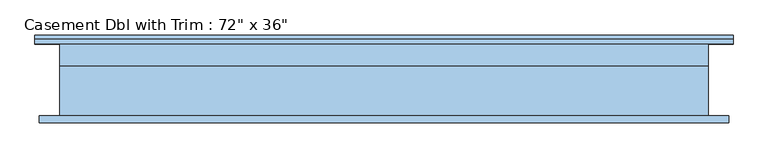
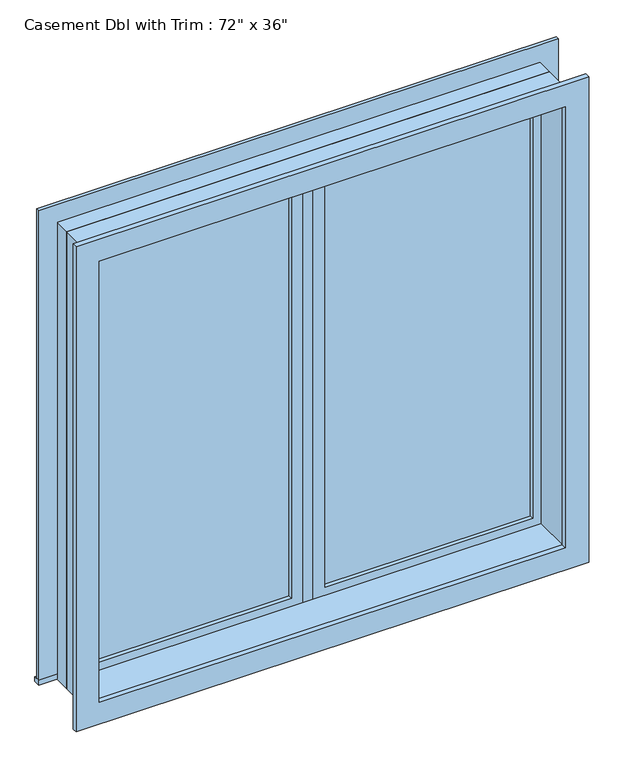
"""IFC4 building model written with IfcOpenShell, lengths in millimetres: window geometry."""

from ifc_helpers import new_model, si_unit, frame, origin, place, context, project, spatial, polyline, outline, extrude, source, transform, mapped, element, save


def window_b085ff8d(model_context):
    return source(origin(), model_context, "Body", "SweptSolid", [
        extrude(outline(polyline([(63.5, 85.725), (850.9, 85.725), (850.9, 73.025), (63.5, 73.025), (63.5, 85.725)])), frame((0.0, 0.0, 1282.7), z_axis=(0.0, 0.0, 1.0), x_axis=(1.0, 0.0, 0.0)), (0.0, 0.0, 1.0), 1701.8),
        extrude(outline(polyline([(3028.95, 19.05), (1238.25, 19.05), (1238.25, 895.35), (3028.95, 895.35), (3028.95, 19.05)]), holes=[polyline([(2984.5, 63.5), (2984.5, 850.9), (1282.7, 850.9), (1282.7, 63.5), (2984.5, 63.5)])]), frame((0.0, 57.15, 0.0), z_axis=(0.0, 1.0, 0.0), x_axis=(0.0, 0.0, 1.0)), (0.0, 0.0, 1.0), 44.45),
        extrude(outline(polyline([(19.05, 57.15), (-19.05, 57.15), (-19.05, 120.65), (19.05, 120.65), (19.05, 57.15)])), frame((0.0, 0.0, 1238.25), z_axis=(0.0, 0.0, 1.0), x_axis=(1.0, 0.0, 0.0)), (0.0, 0.0, 1.0), 1790.7),
        extrude(outline(polyline([(-984.25, 146.05), (984.25, 146.05), (984.25, 120.65), (-984.25, 120.65), (-984.25, 146.05)])), frame((0.0, 0.0, 1219.2), z_axis=(0.0, 0.0, 1.0), x_axis=(1.0, 0.0, 0.0)), (0.0, 0.0, 1.0), 19.05),
        extrude(outline(polyline([(3028.95, -895.35), (3028.95, 895.35), (1238.25, 895.35), (1238.25, 984.25), (3117.85, 984.25), (3117.85, -984.25), (1238.25, -984.25), (1238.25, -895.35), (3028.95, -895.35)])), frame((0.0, 120.65, 0.0), z_axis=(0.0, 1.0, 0.0), x_axis=(0.0, 0.0, 1.0)), (0.0, 0.0, 1.0), 12.7),
        extrude(outline(polyline([(3105.15, 971.55), (3105.15, -971.55), (1162.05, -971.55), (1162.05, 971.55), (3105.15, 971.55)]), holes=[polyline([(3016.25, 882.65), (1250.95, 882.65), (1250.95, -882.65), (3016.25, -882.65), (3016.25, 882.65)])]), frame((0.0, -101.6, 0.0), z_axis=(0.0, 1.0, 0.0), x_axis=(0.0, 0.0, 1.0)), (0.0, 0.0, 1.0), 19.05),
        extrude(outline(polyline([(-63.5, 73.025), (-850.9, 73.025), (-850.9, 85.725), (-63.5, 85.725), (-63.5, 73.025)])), frame((0.0, 0.0, 1282.7), z_axis=(0.0, 0.0, 1.0), x_axis=(1.0, 0.0, 0.0)), (0.0, 0.0, 1.0), 1701.8),
        extrude(outline(polyline([(3028.95, -895.35), (1238.25, -895.35), (1238.25, -19.05), (3028.95, -19.05), (3028.95, -895.35)]), holes=[polyline([(2984.5, -850.9), (2984.5, -63.5), (1282.7, -63.5), (1282.7, -850.9), (2984.5, -850.9)])]), frame((0.0, 57.15, 0.0), z_axis=(0.0, 1.0, 0.0), x_axis=(0.0, 0.0, 1.0)), (0.0, 0.0, 1.0), 44.45),
        extrude(outline(polyline([(3048.0, -914.4), (1219.2, -914.4), (1219.2, 914.4), (3048.0, 914.4), (3048.0, -914.4)]), holes=[polyline([(3016.25, -882.65), (3016.25, 882.65), (1250.95, 882.65), (1250.95, -882.65), (3016.25, -882.65)])]), frame((0.0, -82.55, 0.0), z_axis=(0.0, 1.0, 0.0), x_axis=(0.0, 0.0, 1.0)), (0.0, 0.0, 1.0), 139.7),
        extrude(outline(polyline([(3048.0, 914.4), (3048.0, -914.4), (1219.2, -914.4), (1219.2, 914.4), (3048.0, 914.4)]), holes=[polyline([(3028.95, 895.35), (1238.25, 895.35), (1238.25, -895.35), (3028.95, -895.35), (3028.95, 895.35)])]), frame((0.0, 57.15, 0.0), z_axis=(0.0, 1.0, 0.0), x_axis=(0.0, 0.0, 1.0)), (0.0, 0.0, 1.0), 63.5),
    ])


if __name__ == "__main__":
    model = new_model("IFC4")
    model_context = context("Model", 3, world=origin())
    ifc_project = project(units=[si_unit("LENGTHUNIT", "METRE", prefix="MILLI")], contexts=[model_context])
    site = spatial("IfcSite", under=ifc_project)
    building = spatial("IfcBuilding", under=site)
    placement = place(None, origin())
    window_shape = window_b085ff8d(model_context)
    element("IfcWindow", 1, ObjectType="Casement Dbl with Trim : 72\" x 36\"", at=placement, inside=building, context=model_context, shape_type="MappedRepresentation", body=[
        mapped(window_shape, transform((0.0, 0.0, 0.0), x_axis=(1.0, 0.0, 0.0), y_axis=(0.0, 1.0, 0.0), z_axis=(0.0, 0.0, 1.0))),
    ])
    save(model, "model.ifc")

# Revit data of these elements
# Type "Casement Dbl with Trim : 72\" x 36\""
#   Type Mark = "11"
#   Construction Type Id = "GSP4R"
#   Assembly Code = "B2020100"
#   Analytic Construction = "1/8 in Pilkington single glazing"
#   Visual Light Transmittance = 0.9
#   Solar Heat Gain Coefficient = 0.78
#   Heat Transfer Coefficient (U) = 0.6496 BTU/(h·ft²·°F)
#   Height = 6' - 0"
#   Default Sill Height = 4' - 0"
#   Trim Projection - Ext. = 0' - 0 1/2"
#   Trim Projection - Int. = 0' - 0 3/4"
#   Trim Width - Exterior = 0' - 3 1/2"
#   Trim Width - Interior = 0' - 3 1/2"
#   Width = 6' - 0"
#   Window Inset = 0' - 0 3/4"
#   Define Thermal Properties by = 1
#   Glass Pane Material = Glass
#   Sash Material = Sash
#   Trim Exterior Material = Trim
#   Trim Interior Material = Trim
#   Wall Closure = (empty or 0)
# Element 1 (IfcWindow, "Casement Dbl with Trim : 72\" x 36\"")
#   Materials on its faces: "Sash", "Trim", "Glass"
# Materials
#   "Glass": class "Glass", colour RGB 0 128 192, transparency 0.75, Description = "Soda Lime Glass", Cost = 0
#   "Sash": class "Wood", colour RGB 224 178 126, transparency 0
#   "Trim": class "Wood", colour RGB 224 178 126, transparency 0
